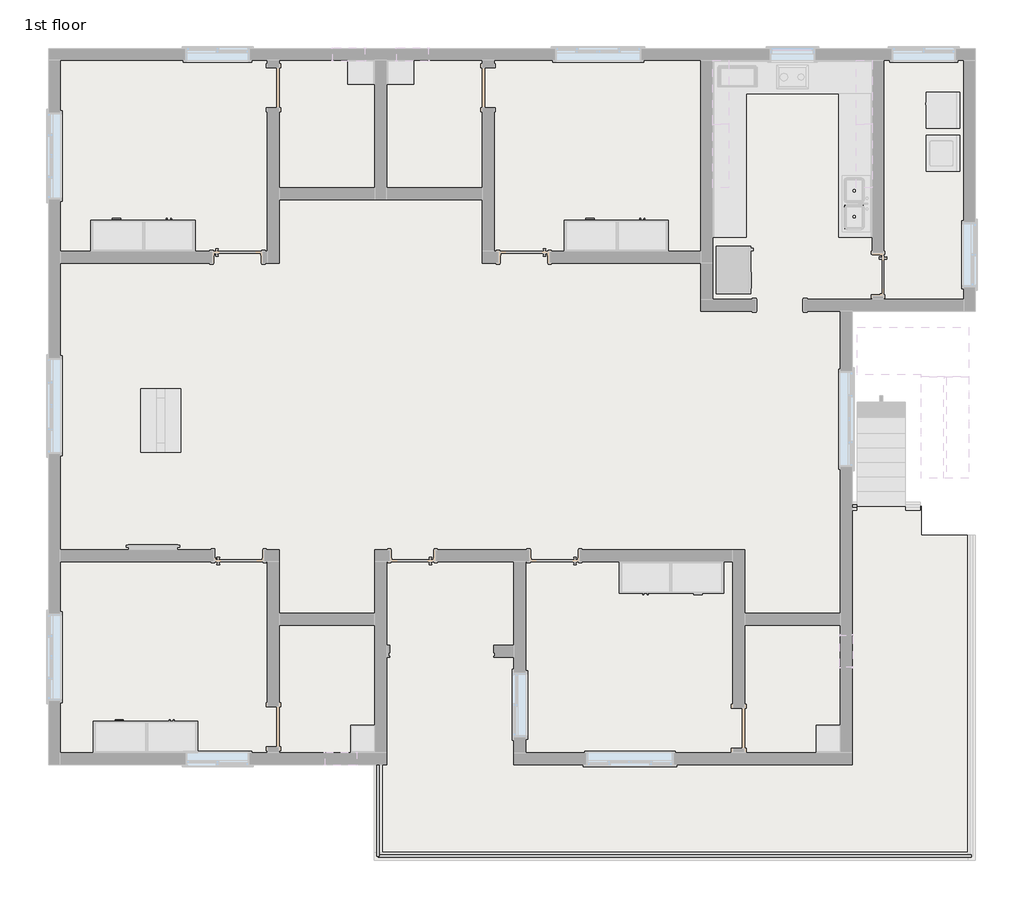
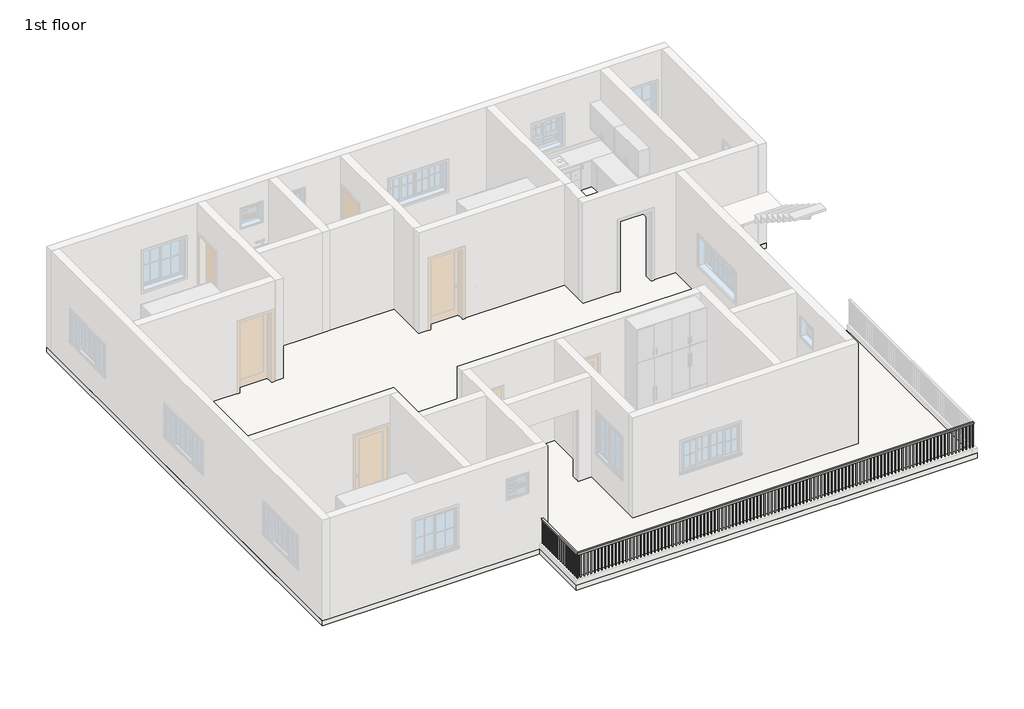
# One storey, part 2 of 4: 3 railings, 1 slab.
"""IFC4 building model written with IfcOpenShell, lengths in millimetres."""

from ifc_helpers import new_model, si_unit, frame, origin, place, context, project, spatial, polyline, outline, extrude, element, save

model = new_model("IFC4")

# Units and contexts
model_context = context("Model", 3, world=origin())
ifc_project = project(units=[si_unit("LENGTHUNIT", "METRE", prefix="MILLI")], contexts=[model_context])

# Site, building, storey
site = spatial("IfcSite", under=ifc_project)
building = spatial("IfcBuilding", under=site)
storey = spatial("IfcBuildingStorey", under=building, Name="1st floor", Elevation=3810.0)

# Railings
placement = place(None, origin())
element("IfcRailing", 1, ObjectType="Handrail - Rectangular", at=placement, inside=storey, context=model_context, shape_type="SweptSolid", body=[
    extrude(outline(polyline([(9648.8260838, -8369.2339187), (9648.8260838, -8420.0339187), (-1717.6739162, -8420.0339187), (-1717.6739162, -8369.2339187), (9648.8260838, -8369.2339187)])), frame((0.0, 0.0, 4673.6), z_axis=(0.0, 0.0, 1.0), x_axis=(1.0, 0.0, 0.0)), (0.0, 0.0, 1.0), 50.8),
    extrude(outline(polyline([(-1619.2489162, -8385.1089187), (-1619.2489162, -8404.1589187), (-1638.2989162, -8404.1589187), (-1638.2989162, -8385.1089187), (-1619.2489162, -8385.1089187)])), frame((0.0, 0.0, 3810.0), z_axis=(0.0, 0.0, 1.0), x_axis=(1.0, 0.0, 0.0)), (0.0, 0.0, 1.0), 863.6),
    extrude(outline(polyline([(-1517.6489162, -8385.1089187), (-1517.6489162, -8404.1589187), (-1536.6989162, -8404.1589187), (-1536.6989162, -8385.1089187), (-1517.6489162, -8385.1089187)])), frame((0.0, 0.0, 3810.0), z_axis=(0.0, 0.0, 1.0), x_axis=(1.0, 0.0, 0.0)), (0.0, 0.0, 1.0), 863.6),
    extrude(outline(polyline([(-1416.0489162, -8385.1089187), (-1416.0489162, -8404.1589187), (-1435.0989162, -8404.1589187), (-1435.0989162, -8385.1089187), (-1416.0489162, -8385.1089187)])), frame((0.0, 0.0, 3810.0), z_axis=(0.0, 0.0, 1.0), x_axis=(1.0, 0.0, 0.0)), (0.0, 0.0, 1.0), 863.6),
    extrude(outline(polyline([(-1314.4489162, -8385.1089187), (-1314.4489162, -8404.1589187), (-1333.4989162, -8404.1589187), (-1333.4989162, -8385.1089187), (-1314.4489162, -8385.1089187)])), frame((0.0, 0.0, 3810.0), z_axis=(0.0, 0.0, 1.0), x_axis=(1.0, 0.0, 0.0)), (0.0, 0.0, 1.0), 863.6),
    extrude(outline(polyline([(-1212.8489162, -8385.1089187), (-1212.8489162, -8404.1589187), (-1231.8989162, -8404.1589187), (-1231.8989162, -8385.1089187), (-1212.8489162, -8385.1089187)])), frame((0.0, 0.0, 3810.0), z_axis=(0.0, 0.0, 1.0), x_axis=(1.0, 0.0, 0.0)), (0.0, 0.0, 1.0), 863.6),
    extrude(outline(polyline([(-1111.2489162, -8385.1089187), (-1111.2489162, -8404.1589187), (-1130.2989162, -8404.1589187), (-1130.2989162, -8385.1089187), (-1111.2489162, -8385.1089187)])), frame((0.0, 0.0, 3810.0), z_axis=(0.0, 0.0, 1.0), x_axis=(1.0, 0.0, 0.0)), (0.0, 0.0, 1.0), 863.6),
    extrude(outline(polyline([(-1009.6489162, -8385.1089187), (-1009.6489162, -8404.1589187), (-1028.6989162, -8404.1589187), (-1028.6989162, -8385.1089187), (-1009.6489162, -8385.1089187)])), frame((0.0, 0.0, 3810.0), z_axis=(0.0, 0.0, 1.0), x_axis=(1.0, 0.0, 0.0)), (0.0, 0.0, 1.0), 863.6),
    extrude(outline(polyline([(-908.0489162, -8385.1089187), (-908.0489162, -8404.1589187), (-927.0989162, -8404.1589187), (-927.0989162, -8385.1089187), (-908.0489162, -8385.1089187)])), frame((0.0, 0.0, 3810.0), z_axis=(0.0, 0.0, 1.0), x_axis=(1.0, 0.0, 0.0)), (0.0, 0.0, 1.0), 863.6),
    extrude(outline(polyline([(-806.4489162, -8385.1089187), (-806.4489162, -8404.1589187), (-825.4989162, -8404.1589187), (-825.4989162, -8385.1089187), (-806.4489162, -8385.1089187)])), frame((0.0, 0.0, 3810.0), z_axis=(0.0, 0.0, 1.0), x_axis=(1.0, 0.0, 0.0)), (0.0, 0.0, 1.0), 863.6),
    extrude(outline(polyline([(-704.8489162, -8385.1089187), (-704.8489162, -8404.1589187), (-723.8989162, -8404.1589187), (-723.8989162, -8385.1089187), (-704.8489162, -8385.1089187)])), frame((0.0, 0.0, 3810.0), z_axis=(0.0, 0.0, 1.0), x_axis=(1.0, 0.0, 0.0)), (0.0, 0.0, 1.0), 863.6),
    extrude(outline(polyline([(-603.2489162, -8385.1089187), (-603.2489162, -8404.1589187), (-622.2989162, -8404.1589187), (-622.2989162, -8385.1089187), (-603.2489162, -8385.1089187)])), frame((0.0, 0.0, 3810.0), z_axis=(0.0, 0.0, 1.0), x_axis=(1.0, 0.0, 0.0)), (0.0, 0.0, 1.0), 863.6),
    extrude(outline(polyline([(-501.6489162, -8385.1089187), (-501.6489162, -8404.1589187), (-520.6989162, -8404.1589187), (-520.6989162, -8385.1089187), (-501.6489162, -8385.1089187)])), frame((0.0, 0.0, 3810.0), z_axis=(0.0, 0.0, 1.0), x_axis=(1.0, 0.0, 0.0)), (0.0, 0.0, 1.0), 863.6),
    extrude(outline(polyline([(-400.0489162, -8385.1089187), (-400.0489162, -8404.1589187), (-419.0989162, -8404.1589187), (-419.0989162, -8385.1089187), (-400.0489162, -8385.1089187)])), frame((0.0, 0.0, 3810.0), z_axis=(0.0, 0.0, 1.0), x_axis=(1.0, 0.0, 0.0)), (0.0, 0.0, 1.0), 863.6),
    extrude(outline(polyline([(-298.4489162, -8385.1089187), (-298.4489162, -8404.1589187), (-317.4989162, -8404.1589187), (-317.4989162, -8385.1089187), (-298.4489162, -8385.1089187)])), frame((0.0, 0.0, 3810.0), z_axis=(0.0, 0.0, 1.0), x_axis=(1.0, 0.0, 0.0)), (0.0, 0.0, 1.0), 863.6),
    extrude(outline(polyline([(-196.8489162, -8385.1089187), (-196.8489162, -8404.1589187), (-215.8989162, -8404.1589187), (-215.8989162, -8385.1089187), (-196.8489162, -8385.1089187)])), frame((0.0, 0.0, 3810.0), z_axis=(0.0, 0.0, 1.0), x_axis=(1.0, 0.0, 0.0)), (0.0, 0.0, 1.0), 863.6),
    extrude(outline(polyline([(-95.2489162, -8385.1089187), (-95.2489162, -8404.1589187), (-114.2989162, -8404.1589187), (-114.2989162, -8385.1089187), (-95.2489162, -8385.1089187)])), frame((0.0, 0.0, 3810.0), z_axis=(0.0, 0.0, 1.0), x_axis=(1.0, 0.0, 0.0)), (0.0, 0.0, 1.0), 863.6),
    extrude(outline(polyline([(6.3510838, -8385.1089187), (6.3510838, -8404.1589187), (-12.6989162, -8404.1589187), (-12.6989162, -8385.1089187), (6.3510838, -8385.1089187)])), frame((0.0, 0.0, 3810.0), z_axis=(0.0, 0.0, 1.0), x_axis=(1.0, 0.0, 0.0)), (0.0, 0.0, 1.0), 863.6),
    extrude(outline(polyline([(107.9510838, -8385.1089187), (107.9510838, -8404.1589187), (88.9010838, -8404.1589187), (88.9010838, -8385.1089187), (107.9510838, -8385.1089187)])), frame((0.0, 0.0, 3810.0), z_axis=(0.0, 0.0, 1.0), x_axis=(1.0, 0.0, 0.0)), (0.0, 0.0, 1.0), 863.6),
    extrude(outline(polyline([(209.5510838, -8385.1089187), (209.5510838, -8404.1589187), (190.5010838, -8404.1589187), (190.5010838, -8385.1089187), (209.5510838, -8385.1089187)])), frame((0.0, 0.0, 3810.0), z_axis=(0.0, 0.0, 1.0), x_axis=(1.0, 0.0, 0.0)), (0.0, 0.0, 1.0), 863.6),
    extrude(outline(polyline([(311.1510838, -8385.1089187), (311.1510838, -8404.1589187), (292.1010838, -8404.1589187), (292.1010838, -8385.1089187), (311.1510838, -8385.1089187)])), frame((0.0, 0.0, 3810.0), z_axis=(0.0, 0.0, 1.0), x_axis=(1.0, 0.0, 0.0)), (0.0, 0.0, 1.0), 863.6),
    extrude(outline(polyline([(412.7510838, -8385.1089187), (412.7510838, -8404.1589187), (393.7010838, -8404.1589187), (393.7010838, -8385.1089187), (412.7510838, -8385.1089187)])), frame((0.0, 0.0, 3810.0), z_axis=(0.0, 0.0, 1.0), x_axis=(1.0, 0.0, 0.0)), (0.0, 0.0, 1.0), 863.6),
    extrude(outline(polyline([(514.3510838, -8385.1089187), (514.3510838, -8404.1589187), (495.3010838, -8404.1589187), (495.3010838, -8385.1089187), (514.3510838, -8385.1089187)])), frame((0.0, 0.0, 3810.0), z_axis=(0.0, 0.0, 1.0), x_axis=(1.0, 0.0, 0.0)), (0.0, 0.0, 1.0), 863.6),
    extrude(outline(polyline([(615.9510838, -8385.1089187), (615.9510838, -8404.1589187), (596.9010838, -8404.1589187), (596.9010838, -8385.1089187), (615.9510838, -8385.1089187)])), frame((0.0, 0.0, 3810.0), z_axis=(0.0, 0.0, 1.0), x_axis=(1.0, 0.0, 0.0)), (0.0, 0.0, 1.0), 863.6),
    extrude(outline(polyline([(717.5510838, -8385.1089187), (717.5510838, -8404.1589187), (698.5010838, -8404.1589187), (698.5010838, -8385.1089187), (717.5510838, -8385.1089187)])), frame((0.0, 0.0, 3810.0), z_axis=(0.0, 0.0, 1.0), x_axis=(1.0, 0.0, 0.0)), (0.0, 0.0, 1.0), 863.6),
    extrude(outline(polyline([(819.1510838, -8385.1089187), (819.1510838, -8404.1589187), (800.1010838, -8404.1589187), (800.1010838, -8385.1089187), (819.1510838, -8385.1089187)])), frame((0.0, 0.0, 3810.0), z_axis=(0.0, 0.0, 1.0), x_axis=(1.0, 0.0, 0.0)), (0.0, 0.0, 1.0), 863.6),
    extrude(outline(polyline([(920.7510838, -8385.1089187), (920.7510838, -8404.1589187), (901.7010838, -8404.1589187), (901.7010838, -8385.1089187), (920.7510838, -8385.1089187)])), frame((0.0, 0.0, 3810.0), z_axis=(0.0, 0.0, 1.0), x_axis=(1.0, 0.0, 0.0)), (0.0, 0.0, 1.0), 863.6),
    extrude(outline(polyline([(1022.3510838, -8385.1089187), (1022.3510838, -8404.1589187), (1003.3010838, -8404.1589187), (1003.3010838, -8385.1089187), (1022.3510838, -8385.1089187)])), frame((0.0, 0.0, 3810.0), z_axis=(0.0, 0.0, 1.0), x_axis=(1.0, 0.0, 0.0)), (0.0, 0.0, 1.0), 863.6),
    extrude(outline(polyline([(1123.9510838, -8385.1089187), (1123.9510838, -8404.1589187), (1104.9010838, -8404.1589187), (1104.9010838, -8385.1089187), (1123.9510838, -8385.1089187)])), frame((0.0, 0.0, 3810.0), z_axis=(0.0, 0.0, 1.0), x_axis=(1.0, 0.0, 0.0)), (0.0, 0.0, 1.0), 863.6),
    extrude(outline(polyline([(1225.5510838, -8385.1089187), (1225.5510838, -8404.1589187), (1206.5010838, -8404.1589187), (1206.5010838, -8385.1089187), (1225.5510838, -8385.1089187)])), frame((0.0, 0.0, 3810.0), z_axis=(0.0, 0.0, 1.0), x_axis=(1.0, 0.0, 0.0)), (0.0, 0.0, 1.0), 863.6),
    extrude(outline(polyline([(1327.1510838, -8385.1089187), (1327.1510838, -8404.1589187), (1308.1010838, -8404.1589187), (1308.1010838, -8385.1089187), (1327.1510838, -8385.1089187)])), frame((0.0, 0.0, 3810.0), z_axis=(0.0, 0.0, 1.0), x_axis=(1.0, 0.0, 0.0)), (0.0, 0.0, 1.0), 863.6),
    extrude(outline(polyline([(1428.7510838, -8385.1089187), (1428.7510838, -8404.1589187), (1409.7010838, -8404.1589187), (1409.7010838, -8385.1089187), (1428.7510838, -8385.1089187)])), frame((0.0, 0.0, 3810.0), z_axis=(0.0, 0.0, 1.0), x_axis=(1.0, 0.0, 0.0)), (0.0, 0.0, 1.0), 863.6),
    extrude(outline(polyline([(1530.3510838, -8385.1089187), (1530.3510838, -8404.1589187), (1511.3010838, -8404.1589187), (1511.3010838, -8385.1089187), (1530.3510838, -8385.1089187)])), frame((0.0, 0.0, 3810.0), z_axis=(0.0, 0.0, 1.0), x_axis=(1.0, 0.0, 0.0)), (0.0, 0.0, 1.0), 863.6),
    extrude(outline(polyline([(1631.9510838, -8385.1089187), (1631.9510838, -8404.1589187), (1612.9010838, -8404.1589187), (1612.9010838, -8385.1089187), (1631.9510838, -8385.1089187)])), frame((0.0, 0.0, 3810.0), z_axis=(0.0, 0.0, 1.0), x_axis=(1.0, 0.0, 0.0)), (0.0, 0.0, 1.0), 863.6),
    extrude(outline(polyline([(1733.5510838, -8385.1089187), (1733.5510838, -8404.1589187), (1714.5010838, -8404.1589187), (1714.5010838, -8385.1089187), (1733.5510838, -8385.1089187)])), frame((0.0, 0.0, 3810.0), z_axis=(0.0, 0.0, 1.0), x_axis=(1.0, 0.0, 0.0)), (0.0, 0.0, 1.0), 863.6),
    extrude(outline(polyline([(1835.1510838, -8385.1089187), (1835.1510838, -8404.1589187), (1816.1010838, -8404.1589187), (1816.1010838, -8385.1089187), (1835.1510838, -8385.1089187)])), frame((0.0, 0.0, 3810.0), z_axis=(0.0, 0.0, 1.0), x_axis=(1.0, 0.0, 0.0)), (0.0, 0.0, 1.0), 863.6),
    extrude(outline(polyline([(1936.7510838, -8385.1089187), (1936.7510838, -8404.1589187), (1917.7010838, -8404.1589187), (1917.7010838, -8385.1089187), (1936.7510838, -8385.1089187)])), frame((0.0, 0.0, 3810.0), z_axis=(0.0, 0.0, 1.0), x_axis=(1.0, 0.0, 0.0)), (0.0, 0.0, 1.0), 863.6),
    extrude(outline(polyline([(2038.3510838, -8385.1089187), (2038.3510838, -8404.1589187), (2019.3010838, -8404.1589187), (2019.3010838, -8385.1089187), (2038.3510838, -8385.1089187)])), frame((0.0, 0.0, 3810.0), z_axis=(0.0, 0.0, 1.0), x_axis=(1.0, 0.0, 0.0)), (0.0, 0.0, 1.0), 863.6),
    extrude(outline(polyline([(2139.9510838, -8385.1089187), (2139.9510838, -8404.1589187), (2120.9010838, -8404.1589187), (2120.9010838, -8385.1089187), (2139.9510838, -8385.1089187)])), frame((0.0, 0.0, 3810.0), z_axis=(0.0, 0.0, 1.0), x_axis=(1.0, 0.0, 0.0)), (0.0, 0.0, 1.0), 863.6),
    extrude(outline(polyline([(2241.5510838, -8385.1089187), (2241.5510838, -8404.1589187), (2222.5010838, -8404.1589187), (2222.5010838, -8385.1089187), (2241.5510838, -8385.1089187)])), frame((0.0, 0.0, 3810.0), z_axis=(0.0, 0.0, 1.0), x_axis=(1.0, 0.0, 0.0)), (0.0, 0.0, 1.0), 863.6),
    extrude(outline(polyline([(2343.1510838, -8385.1089187), (2343.1510838, -8404.1589187), (2324.1010838, -8404.1589187), (2324.1010838, -8385.1089187), (2343.1510838, -8385.1089187)])), frame((0.0, 0.0, 3810.0), z_axis=(0.0, 0.0, 1.0), x_axis=(1.0, 0.0, 0.0)), (0.0, 0.0, 1.0), 863.6),
    extrude(outline(polyline([(2444.7510838, -8385.1089187), (2444.7510838, -8404.1589187), (2425.7010838, -8404.1589187), (2425.7010838, -8385.1089187), (2444.7510838, -8385.1089187)])), frame((0.0, 0.0, 3810.0), z_axis=(0.0, 0.0, 1.0), x_axis=(1.0, 0.0, 0.0)), (0.0, 0.0, 1.0), 863.6),
    extrude(outline(polyline([(2546.3510838, -8385.1089187), (2546.3510838, -8404.1589187), (2527.3010838, -8404.1589187), (2527.3010838, -8385.1089187), (2546.3510838, -8385.1089187)])), frame((0.0, 0.0, 3810.0), z_axis=(0.0, 0.0, 1.0), x_axis=(1.0, 0.0, 0.0)), (0.0, 0.0, 1.0), 863.6),
    extrude(outline(polyline([(2647.9510838, -8385.1089187), (2647.9510838, -8404.1589187), (2628.9010838, -8404.1589187), (2628.9010838, -8385.1089187), (2647.9510838, -8385.1089187)])), frame((0.0, 0.0, 3810.0), z_axis=(0.0, 0.0, 1.0), x_axis=(1.0, 0.0, 0.0)), (0.0, 0.0, 1.0), 863.6),
    extrude(outline(polyline([(2749.5510838, -8385.1089187), (2749.5510838, -8404.1589187), (2730.5010838, -8404.1589187), (2730.5010838, -8385.1089187), (2749.5510838, -8385.1089187)])), frame((0.0, 0.0, 3810.0), z_axis=(0.0, 0.0, 1.0), x_axis=(1.0, 0.0, 0.0)), (0.0, 0.0, 1.0), 863.6),
    extrude(outline(polyline([(2851.1510838, -8385.1089187), (2851.1510838, -8404.1589187), (2832.1010838, -8404.1589187), (2832.1010838, -8385.1089187), (2851.1510838, -8385.1089187)])), frame((0.0, 0.0, 3810.0), z_axis=(0.0, 0.0, 1.0), x_axis=(1.0, 0.0, 0.0)), (0.0, 0.0, 1.0), 863.6),
    extrude(outline(polyline([(2952.7510838, -8385.1089187), (2952.7510838, -8404.1589187), (2933.7010838, -8404.1589187), (2933.7010838, -8385.1089187), (2952.7510838, -8385.1089187)])), frame((0.0, 0.0, 3810.0), z_axis=(0.0, 0.0, 1.0), x_axis=(1.0, 0.0, 0.0)), (0.0, 0.0, 1.0), 863.6),
    extrude(outline(polyline([(3054.3510838, -8385.1089187), (3054.3510838, -8404.1589187), (3035.3010838, -8404.1589187), (3035.3010838, -8385.1089187), (3054.3510838, -8385.1089187)])), frame((0.0, 0.0, 3810.0), z_axis=(0.0, 0.0, 1.0), x_axis=(1.0, 0.0, 0.0)), (0.0, 0.0, 1.0), 863.6),
    extrude(outline(polyline([(3155.9510838, -8385.1089187), (3155.9510838, -8404.1589187), (3136.9010838, -8404.1589187), (3136.9010838, -8385.1089187), (3155.9510838, -8385.1089187)])), frame((0.0, 0.0, 3810.0), z_axis=(0.0, 0.0, 1.0), x_axis=(1.0, 0.0, 0.0)), (0.0, 0.0, 1.0), 863.6),
    extrude(outline(polyline([(3257.5510838, -8385.1089187), (3257.5510838, -8404.1589187), (3238.5010838, -8404.1589187), (3238.5010838, -8385.1089187), (3257.5510838, -8385.1089187)])), frame((0.0, 0.0, 3810.0), z_axis=(0.0, 0.0, 1.0), x_axis=(1.0, 0.0, 0.0)), (0.0, 0.0, 1.0), 863.6),
    extrude(outline(polyline([(3359.1510838, -8385.1089187), (3359.1510838, -8404.1589187), (3340.1010838, -8404.1589187), (3340.1010838, -8385.1089187), (3359.1510838, -8385.1089187)])), frame((0.0, 0.0, 3810.0), z_axis=(0.0, 0.0, 1.0), x_axis=(1.0, 0.0, 0.0)), (0.0, 0.0, 1.0), 863.6),
    extrude(outline(polyline([(3460.7510838, -8385.1089187), (3460.7510838, -8404.1589187), (3441.7010838, -8404.1589187), (3441.7010838, -8385.1089187), (3460.7510838, -8385.1089187)])), frame((0.0, 0.0, 3810.0), z_axis=(0.0, 0.0, 1.0), x_axis=(1.0, 0.0, 0.0)), (0.0, 0.0, 1.0), 863.6),
    extrude(outline(polyline([(3562.3510838, -8385.1089187), (3562.3510838, -8404.1589187), (3543.3010838, -8404.1589187), (3543.3010838, -8385.1089187), (3562.3510838, -8385.1089187)])), frame((0.0, 0.0, 3810.0), z_axis=(0.0, 0.0, 1.0), x_axis=(1.0, 0.0, 0.0)), (0.0, 0.0, 1.0), 863.6),
    extrude(outline(polyline([(3663.9510838, -8385.1089187), (3663.9510838, -8404.1589187), (3644.9010838, -8404.1589187), (3644.9010838, -8385.1089187), (3663.9510838, -8385.1089187)])), frame((0.0, 0.0, 3810.0), z_axis=(0.0, 0.0, 1.0), x_axis=(1.0, 0.0, 0.0)), (0.0, 0.0, 1.0), 863.6),
    extrude(outline(polyline([(3765.5510838, -8385.1089187), (3765.5510838, -8404.1589187), (3746.5010838, -8404.1589187), (3746.5010838, -8385.1089187), (3765.5510838, -8385.1089187)])), frame((0.0, 0.0, 3810.0), z_axis=(0.0, 0.0, 1.0), x_axis=(1.0, 0.0, 0.0)), (0.0, 0.0, 1.0), 863.6),
    extrude(outline(polyline([(3867.1510838, -8385.1089187), (3867.1510838, -8404.1589187), (3848.1010838, -8404.1589187), (3848.1010838, -8385.1089187), (3867.1510838, -8385.1089187)])), frame((0.0, 0.0, 3810.0), z_axis=(0.0, 0.0, 1.0), x_axis=(1.0, 0.0, 0.0)), (0.0, 0.0, 1.0), 863.6),
    extrude(outline(polyline([(3968.7510838, -8385.1089187), (3968.7510838, -8404.1589187), (3949.7010838, -8404.1589187), (3949.7010838, -8385.1089187), (3968.7510838, -8385.1089187)])), frame((0.0, 0.0, 3810.0), z_axis=(0.0, 0.0, 1.0), x_axis=(1.0, 0.0, 0.0)), (0.0, 0.0, 1.0), 863.6),
    extrude(outline(polyline([(4070.3510838, -8385.1089187), (4070.3510838, -8404.1589187), (4051.3010838, -8404.1589187), (4051.3010838, -8385.1089187), (4070.3510838, -8385.1089187)])), frame((0.0, 0.0, 3810.0), z_axis=(0.0, 0.0, 1.0), x_axis=(1.0, 0.0, 0.0)), (0.0, 0.0, 1.0), 863.6),
    extrude(outline(polyline([(4171.9510838, -8385.1089187), (4171.9510838, -8404.1589187), (4152.9010838, -8404.1589187), (4152.9010838, -8385.1089187), (4171.9510838, -8385.1089187)])), frame((0.0, 0.0, 3810.0), z_axis=(0.0, 0.0, 1.0), x_axis=(1.0, 0.0, 0.0)), (0.0, 0.0, 1.0), 863.6),
    extrude(outline(polyline([(4273.5510838, -8385.1089187), (4273.5510838, -8404.1589187), (4254.5010838, -8404.1589187), (4254.5010838, -8385.1089187), (4273.5510838, -8385.1089187)])), frame((0.0, 0.0, 3810.0), z_axis=(0.0, 0.0, 1.0), x_axis=(1.0, 0.0, 0.0)), (0.0, 0.0, 1.0), 863.6),
    extrude(outline(polyline([(4375.1510838, -8385.1089187), (4375.1510838, -8404.1589187), (4356.1010838, -8404.1589187), (4356.1010838, -8385.1089187), (4375.1510838, -8385.1089187)])), frame((0.0, 0.0, 3810.0), z_axis=(0.0, 0.0, 1.0), x_axis=(1.0, 0.0, 0.0)), (0.0, 0.0, 1.0), 863.6),
    extrude(outline(polyline([(4476.7510838, -8385.1089187), (4476.7510838, -8404.1589187), (4457.7010838, -8404.1589187), (4457.7010838, -8385.1089187), (4476.7510838, -8385.1089187)])), frame((0.0, 0.0, 3810.0), z_axis=(0.0, 0.0, 1.0), x_axis=(1.0, 0.0, 0.0)), (0.0, 0.0, 1.0), 863.6),
    extrude(outline(polyline([(4578.3510838, -8385.1089187), (4578.3510838, -8404.1589187), (4559.3010838, -8404.1589187), (4559.3010838, -8385.1089187), (4578.3510838, -8385.1089187)])), frame((0.0, 0.0, 3810.0), z_axis=(0.0, 0.0, 1.0), x_axis=(1.0, 0.0, 0.0)), (0.0, 0.0, 1.0), 863.6),
    extrude(outline(polyline([(4679.9510838, -8385.1089187), (4679.9510838, -8404.1589187), (4660.9010838, -8404.1589187), (4660.9010838, -8385.1089187), (4679.9510838, -8385.1089187)])), frame((0.0, 0.0, 3810.0), z_axis=(0.0, 0.0, 1.0), x_axis=(1.0, 0.0, 0.0)), (0.0, 0.0, 1.0), 863.6),
    extrude(outline(polyline([(4781.5510838, -8385.1089187), (4781.5510838, -8404.1589187), (4762.5010838, -8404.1589187), (4762.5010838, -8385.1089187), (4781.5510838, -8385.1089187)])), frame((0.0, 0.0, 3810.0), z_axis=(0.0, 0.0, 1.0), x_axis=(1.0, 0.0, 0.0)), (0.0, 0.0, 1.0), 863.6),
    extrude(outline(polyline([(4883.1510838, -8385.1089187), (4883.1510838, -8404.1589187), (4864.1010838, -8404.1589187), (4864.1010838, -8385.1089187), (4883.1510838, -8385.1089187)])), frame((0.0, 0.0, 3810.0), z_axis=(0.0, 0.0, 1.0), x_axis=(1.0, 0.0, 0.0)), (0.0, 0.0, 1.0), 863.6),
    extrude(outline(polyline([(4984.7510838, -8385.1089187), (4984.7510838, -8404.1589187), (4965.7010838, -8404.1589187), (4965.7010838, -8385.1089187), (4984.7510838, -8385.1089187)])), frame((0.0, 0.0, 3810.0), z_axis=(0.0, 0.0, 1.0), x_axis=(1.0, 0.0, 0.0)), (0.0, 0.0, 1.0), 863.6),
    extrude(outline(polyline([(5086.3510838, -8385.1089187), (5086.3510838, -8404.1589187), (5067.3010838, -8404.1589187), (5067.3010838, -8385.1089187), (5086.3510838, -8385.1089187)])), frame((0.0, 0.0, 3810.0), z_axis=(0.0, 0.0, 1.0), x_axis=(1.0, 0.0, 0.0)), (0.0, 0.0, 1.0), 863.6),
    extrude(outline(polyline([(5187.9510838, -8385.1089187), (5187.9510838, -8404.1589187), (5168.9010838, -8404.1589187), (5168.9010838, -8385.1089187), (5187.9510838, -8385.1089187)])), frame((0.0, 0.0, 3810.0), z_axis=(0.0, 0.0, 1.0), x_axis=(1.0, 0.0, 0.0)), (0.0, 0.0, 1.0), 863.6),
    extrude(outline(polyline([(5289.5510838, -8385.1089187), (5289.5510838, -8404.1589187), (5270.5010838, -8404.1589187), (5270.5010838, -8385.1089187), (5289.5510838, -8385.1089187)])), frame((0.0, 0.0, 3810.0), z_axis=(0.0, 0.0, 1.0), x_axis=(1.0, 0.0, 0.0)), (0.0, 0.0, 1.0), 863.6),
    extrude(outline(polyline([(5391.1510838, -8385.1089187), (5391.1510838, -8404.1589187), (5372.1010838, -8404.1589187), (5372.1010838, -8385.1089187), (5391.1510838, -8385.1089187)])), frame((0.0, 0.0, 3810.0), z_axis=(0.0, 0.0, 1.0), x_axis=(1.0, 0.0, 0.0)), (0.0, 0.0, 1.0), 863.6),
    extrude(outline(polyline([(5492.7510838, -8385.1089187), (5492.7510838, -8404.1589187), (5473.7010838, -8404.1589187), (5473.7010838, -8385.1089187), (5492.7510838, -8385.1089187)])), frame((0.0, 0.0, 3810.0), z_axis=(0.0, 0.0, 1.0), x_axis=(1.0, 0.0, 0.0)), (0.0, 0.0, 1.0), 863.6),
    extrude(outline(polyline([(5594.3510838, -8385.1089187), (5594.3510838, -8404.1589187), (5575.3010838, -8404.1589187), (5575.3010838, -8385.1089187), (5594.3510838, -8385.1089187)])), frame((0.0, 0.0, 3810.0), z_axis=(0.0, 0.0, 1.0), x_axis=(1.0, 0.0, 0.0)), (0.0, 0.0, 1.0), 863.6),
    extrude(outline(polyline([(5695.9510838, -8385.1089187), (5695.9510838, -8404.1589187), (5676.9010838, -8404.1589187), (5676.9010838, -8385.1089187), (5695.9510838, -8385.1089187)])), frame((0.0, 0.0, 3810.0), z_axis=(0.0, 0.0, 1.0), x_axis=(1.0, 0.0, 0.0)), (0.0, 0.0, 1.0), 863.6),
    extrude(outline(polyline([(5797.5510838, -8385.1089187), (5797.5510838, -8404.1589187), (5778.5010838, -8404.1589187), (5778.5010838, -8385.1089187), (5797.5510838, -8385.1089187)])), frame((0.0, 0.0, 3810.0), z_axis=(0.0, 0.0, 1.0), x_axis=(1.0, 0.0, 0.0)), (0.0, 0.0, 1.0), 863.6),
    extrude(outline(polyline([(5899.1510838, -8385.1089187), (5899.1510838, -8404.1589187), (5880.1010838, -8404.1589187), (5880.1010838, -8385.1089187), (5899.1510838, -8385.1089187)])), frame((0.0, 0.0, 3810.0), z_axis=(0.0, 0.0, 1.0), x_axis=(1.0, 0.0, 0.0)), (0.0, 0.0, 1.0), 863.6),
    extrude(outline(polyline([(6000.7510838, -8385.1089187), (6000.7510838, -8404.1589187), (5981.7010838, -8404.1589187), (5981.7010838, -8385.1089187), (6000.7510838, -8385.1089187)])), frame((0.0, 0.0, 3810.0), z_axis=(0.0, 0.0, 1.0), x_axis=(1.0, 0.0, 0.0)), (0.0, 0.0, 1.0), 863.6),
    extrude(outline(polyline([(6102.3510838, -8385.1089187), (6102.3510838, -8404.1589187), (6083.3010838, -8404.1589187), (6083.3010838, -8385.1089187), (6102.3510838, -8385.1089187)])), frame((0.0, 0.0, 3810.0), z_axis=(0.0, 0.0, 1.0), x_axis=(1.0, 0.0, 0.0)), (0.0, 0.0, 1.0), 863.6),
    extrude(outline(polyline([(6203.9510838, -8385.1089187), (6203.9510838, -8404.1589187), (6184.9010838, -8404.1589187), (6184.9010838, -8385.1089187), (6203.9510838, -8385.1089187)])), frame((0.0, 0.0, 3810.0), z_axis=(0.0, 0.0, 1.0), x_axis=(1.0, 0.0, 0.0)), (0.0, 0.0, 1.0), 863.6),
    extrude(outline(polyline([(6305.5510838, -8385.1089187), (6305.5510838, -8404.1589187), (6286.5010838, -8404.1589187), (6286.5010838, -8385.1089187), (6305.5510838, -8385.1089187)])), frame((0.0, 0.0, 3810.0), z_axis=(0.0, 0.0, 1.0), x_axis=(1.0, 0.0, 0.0)), (0.0, 0.0, 1.0), 863.6),
    extrude(outline(polyline([(6407.1510838, -8385.1089187), (6407.1510838, -8404.1589187), (6388.1010838, -8404.1589187), (6388.1010838, -8385.1089187), (6407.1510838, -8385.1089187)])), frame((0.0, 0.0, 3810.0), z_axis=(0.0, 0.0, 1.0), x_axis=(1.0, 0.0, 0.0)), (0.0, 0.0, 1.0), 863.6),
    extrude(outline(polyline([(6508.7510838, -8385.1089187), (6508.7510838, -8404.1589187), (6489.7010838, -8404.1589187), (6489.7010838, -8385.1089187), (6508.7510838, -8385.1089187)])), frame((0.0, 0.0, 3810.0), z_axis=(0.0, 0.0, 1.0), x_axis=(1.0, 0.0, 0.0)), (0.0, 0.0, 1.0), 863.6),
    extrude(outline(polyline([(6610.3510838, -8385.1089187), (6610.3510838, -8404.1589187), (6591.3010838, -8404.1589187), (6591.3010838, -8385.1089187), (6610.3510838, -8385.1089187)])), frame((0.0, 0.0, 3810.0), z_axis=(0.0, 0.0, 1.0), x_axis=(1.0, 0.0, 0.0)), (0.0, 0.0, 1.0), 863.6),
    extrude(outline(polyline([(6711.9510838, -8385.1089187), (6711.9510838, -8404.1589187), (6692.9010838, -8404.1589187), (6692.9010838, -8385.1089187), (6711.9510838, -8385.1089187)])), frame((0.0, 0.0, 3810.0), z_axis=(0.0, 0.0, 1.0), x_axis=(1.0, 0.0, 0.0)), (0.0, 0.0, 1.0), 863.6),
    extrude(outline(polyline([(6813.5510838, -8385.1089187), (6813.5510838, -8404.1589187), (6794.5010838, -8404.1589187), (6794.5010838, -8385.1089187), (6813.5510838, -8385.1089187)])), frame((0.0, 0.0, 3810.0), z_axis=(0.0, 0.0, 1.0), x_axis=(1.0, 0.0, 0.0)), (0.0, 0.0, 1.0), 863.6),
    extrude(outline(polyline([(6915.1510838, -8385.1089187), (6915.1510838, -8404.1589187), (6896.1010838, -8404.1589187), (6896.1010838, -8385.1089187), (6915.1510838, -8385.1089187)])), frame((0.0, 0.0, 3810.0), z_axis=(0.0, 0.0, 1.0), x_axis=(1.0, 0.0, 0.0)), (0.0, 0.0, 1.0), 863.6),
    extrude(outline(polyline([(7016.7510838, -8385.1089187), (7016.7510838, -8404.1589187), (6997.7010838, -8404.1589187), (6997.7010838, -8385.1089187), (7016.7510838, -8385.1089187)])), frame((0.0, 0.0, 3810.0), z_axis=(0.0, 0.0, 1.0), x_axis=(1.0, 0.0, 0.0)), (0.0, 0.0, 1.0), 863.6),
    extrude(outline(polyline([(7118.3510838, -8385.1089187), (7118.3510838, -8404.1589187), (7099.3010838, -8404.1589187), (7099.3010838, -8385.1089187), (7118.3510838, -8385.1089187)])), frame((0.0, 0.0, 3810.0), z_axis=(0.0, 0.0, 1.0), x_axis=(1.0, 0.0, 0.0)), (0.0, 0.0, 1.0), 863.6),
    extrude(outline(polyline([(7219.9510838, -8385.1089187), (7219.9510838, -8404.1589187), (7200.9010838, -8404.1589187), (7200.9010838, -8385.1089187), (7219.9510838, -8385.1089187)])), frame((0.0, 0.0, 3810.0), z_axis=(0.0, 0.0, 1.0), x_axis=(1.0, 0.0, 0.0)), (0.0, 0.0, 1.0), 863.6),
    extrude(outline(polyline([(7321.5510838, -8385.1089187), (7321.5510838, -8404.1589187), (7302.5010838, -8404.1589187), (7302.5010838, -8385.1089187), (7321.5510838, -8385.1089187)])), frame((0.0, 0.0, 3810.0), z_axis=(0.0, 0.0, 1.0), x_axis=(1.0, 0.0, 0.0)), (0.0, 0.0, 1.0), 863.6),
    extrude(outline(polyline([(7423.1510838, -8385.1089187), (7423.1510838, -8404.1589187), (7404.1010838, -8404.1589187), (7404.1010838, -8385.1089187), (7423.1510838, -8385.1089187)])), frame((0.0, 0.0, 3810.0), z_axis=(0.0, 0.0, 1.0), x_axis=(1.0, 0.0, 0.0)), (0.0, 0.0, 1.0), 863.6),
    extrude(outline(polyline([(7524.7510838, -8385.1089187), (7524.7510838, -8404.1589187), (7505.7010838, -8404.1589187), (7505.7010838, -8385.1089187), (7524.7510838, -8385.1089187)])), frame((0.0, 0.0, 3810.0), z_axis=(0.0, 0.0, 1.0), x_axis=(1.0, 0.0, 0.0)), (0.0, 0.0, 1.0), 863.6),
    extrude(outline(polyline([(7626.3510838, -8385.1089187), (7626.3510838, -8404.1589187), (7607.3010838, -8404.1589187), (7607.3010838, -8385.1089187), (7626.3510838, -8385.1089187)])), frame((0.0, 0.0, 3810.0), z_axis=(0.0, 0.0, 1.0), x_axis=(1.0, 0.0, 0.0)), (0.0, 0.0, 1.0), 863.6),
    extrude(outline(polyline([(7727.9510838, -8385.1089187), (7727.9510838, -8404.1589187), (7708.9010838, -8404.1589187), (7708.9010838, -8385.1089187), (7727.9510838, -8385.1089187)])), frame((0.0, 0.0, 3810.0), z_axis=(0.0, 0.0, 1.0), x_axis=(1.0, 0.0, 0.0)), (0.0, 0.0, 1.0), 863.6),
    extrude(outline(polyline([(7829.5510838, -8385.1089187), (7829.5510838, -8404.1589187), (7810.5010838, -8404.1589187), (7810.5010838, -8385.1089187), (7829.5510838, -8385.1089187)])), frame((0.0, 0.0, 3810.0), z_axis=(0.0, 0.0, 1.0), x_axis=(1.0, 0.0, 0.0)), (0.0, 0.0, 1.0), 863.6),
    extrude(outline(polyline([(7931.1510838, -8385.1089187), (7931.1510838, -8404.1589187), (7912.1010838, -8404.1589187), (7912.1010838, -8385.1089187), (7931.1510838, -8385.1089187)])), frame((0.0, 0.0, 3810.0), z_axis=(0.0, 0.0, 1.0), x_axis=(1.0, 0.0, 0.0)), (0.0, 0.0, 1.0), 863.6),
    extrude(outline(polyline([(8032.7510838, -8385.1089187), (8032.7510838, -8404.1589187), (8013.7010838, -8404.1589187), (8013.7010838, -8385.1089187), (8032.7510838, -8385.1089187)])), frame((0.0, 0.0, 3810.0), z_axis=(0.0, 0.0, 1.0), x_axis=(1.0, 0.0, 0.0)), (0.0, 0.0, 1.0), 863.6),
    extrude(outline(polyline([(8134.3510838, -8385.1089187), (8134.3510838, -8404.1589187), (8115.3010838, -8404.1589187), (8115.3010838, -8385.1089187), (8134.3510838, -8385.1089187)])), frame((0.0, 0.0, 3810.0), z_axis=(0.0, 0.0, 1.0), x_axis=(1.0, 0.0, 0.0)), (0.0, 0.0, 1.0), 863.6),
    extrude(outline(polyline([(8235.9510838, -8385.1089187), (8235.9510838, -8404.1589187), (8216.9010838, -8404.1589187), (8216.9010838, -8385.1089187), (8235.9510838, -8385.1089187)])), frame((0.0, 0.0, 3810.0), z_axis=(0.0, 0.0, 1.0), x_axis=(1.0, 0.0, 0.0)), (0.0, 0.0, 1.0), 863.6),
    extrude(outline(polyline([(8337.5510838, -8385.1089187), (8337.5510838, -8404.1589187), (8318.5010838, -8404.1589187), (8318.5010838, -8385.1089187), (8337.5510838, -8385.1089187)])), frame((0.0, 0.0, 3810.0), z_axis=(0.0, 0.0, 1.0), x_axis=(1.0, 0.0, 0.0)), (0.0, 0.0, 1.0), 863.6),
    extrude(outline(polyline([(8439.1510838, -8385.1089187), (8439.1510838, -8404.1589187), (8420.1010838, -8404.1589187), (8420.1010838, -8385.1089187), (8439.1510838, -8385.1089187)])), frame((0.0, 0.0, 3810.0), z_axis=(0.0, 0.0, 1.0), x_axis=(1.0, 0.0, 0.0)), (0.0, 0.0, 1.0), 863.6),
    extrude(outline(polyline([(8540.7510838, -8385.1089187), (8540.7510838, -8404.1589187), (8521.7010838, -8404.1589187), (8521.7010838, -8385.1089187), (8540.7510838, -8385.1089187)])), frame((0.0, 0.0, 3810.0), z_axis=(0.0, 0.0, 1.0), x_axis=(1.0, 0.0, 0.0)), (0.0, 0.0, 1.0), 863.6),
    extrude(outline(polyline([(8642.3510838, -8385.1089187), (8642.3510838, -8404.1589187), (8623.3010838, -8404.1589187), (8623.3010838, -8385.1089187), (8642.3510838, -8385.1089187)])), frame((0.0, 0.0, 3810.0), z_axis=(0.0, 0.0, 1.0), x_axis=(1.0, 0.0, 0.0)), (0.0, 0.0, 1.0), 863.6),
    extrude(outline(polyline([(8743.9510838, -8385.1089187), (8743.9510838, -8404.1589187), (8724.9010838, -8404.1589187), (8724.9010838, -8385.1089187), (8743.9510838, -8385.1089187)])), frame((0.0, 0.0, 3810.0), z_axis=(0.0, 0.0, 1.0), x_axis=(1.0, 0.0, 0.0)), (0.0, 0.0, 1.0), 863.6),
    extrude(outline(polyline([(8845.5510838, -8385.1089187), (8845.5510838, -8404.1589187), (8826.5010838, -8404.1589187), (8826.5010838, -8385.1089187), (8845.5510838, -8385.1089187)])), frame((0.0, 0.0, 3810.0), z_axis=(0.0, 0.0, 1.0), x_axis=(1.0, 0.0, 0.0)), (0.0, 0.0, 1.0), 863.6),
    extrude(outline(polyline([(8947.1510838, -8385.1089187), (8947.1510838, -8404.1589187), (8928.1010838, -8404.1589187), (8928.1010838, -8385.1089187), (8947.1510838, -8385.1089187)])), frame((0.0, 0.0, 3810.0), z_axis=(0.0, 0.0, 1.0), x_axis=(1.0, 0.0, 0.0)), (0.0, 0.0, 1.0), 863.6),
    extrude(outline(polyline([(9048.7510838, -8385.1089187), (9048.7510838, -8404.1589187), (9029.7010838, -8404.1589187), (9029.7010838, -8385.1089187), (9048.7510838, -8385.1089187)])), frame((0.0, 0.0, 3810.0), z_axis=(0.0, 0.0, 1.0), x_axis=(1.0, 0.0, 0.0)), (0.0, 0.0, 1.0), 863.6),
    extrude(outline(polyline([(9150.3510838, -8385.1089187), (9150.3510838, -8404.1589187), (9131.3010838, -8404.1589187), (9131.3010838, -8385.1089187), (9150.3510838, -8385.1089187)])), frame((0.0, 0.0, 3810.0), z_axis=(0.0, 0.0, 1.0), x_axis=(1.0, 0.0, 0.0)), (0.0, 0.0, 1.0), 863.6),
    extrude(outline(polyline([(9251.9510838, -8385.1089187), (9251.9510838, -8404.1589187), (9232.9010838, -8404.1589187), (9232.9010838, -8385.1089187), (9251.9510838, -8385.1089187)])), frame((0.0, 0.0, 3810.0), z_axis=(0.0, 0.0, 1.0), x_axis=(1.0, 0.0, 0.0)), (0.0, 0.0, 1.0), 863.6),
    extrude(outline(polyline([(9353.5510838, -8385.1089187), (9353.5510838, -8404.1589187), (9334.5010838, -8404.1589187), (9334.5010838, -8385.1089187), (9353.5510838, -8385.1089187)])), frame((0.0, 0.0, 3810.0), z_axis=(0.0, 0.0, 1.0), x_axis=(1.0, 0.0, 0.0)), (0.0, 0.0, 1.0), 863.6),
    extrude(outline(polyline([(9455.1510838, -8385.1089187), (9455.1510838, -8404.1589187), (9436.1010838, -8404.1589187), (9436.1010838, -8385.1089187), (9455.1510838, -8385.1089187)])), frame((0.0, 0.0, 3810.0), z_axis=(0.0, 0.0, 1.0), x_axis=(1.0, 0.0, 0.0)), (0.0, 0.0, 1.0), 863.6),
    extrude(outline(polyline([(9556.7510838, -8385.1089187), (9556.7510838, -8404.1589187), (9537.7010838, -8404.1589187), (9537.7010838, -8385.1089187), (9556.7510838, -8385.1089187)])), frame((0.0, 0.0, 3810.0), z_axis=(0.0, 0.0, 1.0), x_axis=(1.0, 0.0, 0.0)), (0.0, 0.0, 1.0), 863.6),
    extrude(outline(polyline([(-1698.6239162, -8385.1089187), (-1698.6239162, -8404.1589187), (-1717.6739162, -8404.1589187), (-1717.6739162, -8385.1089187), (-1698.6239162, -8385.1089187)])), frame((0.0, 0.0, 3810.0), z_axis=(0.0, 0.0, 1.0), x_axis=(1.0, 0.0, 0.0)), (0.0, 0.0, 1.0), 863.6),
    extrude(outline(polyline([(9648.8260838, -8385.1089187), (9648.8260838, -8404.1589187), (9629.7760838, -8404.1589187), (9629.7760838, -8385.1089187), (9648.8260838, -8385.1089187)])), frame((0.0, 0.0, 3810.0), z_axis=(0.0, 0.0, 1.0), x_axis=(1.0, 0.0, 0.0)), (0.0, 0.0, 1.0), 863.6),
])
element("IfcRailing", 2, ObjectType="Handrail - Rectangular", at=placement, inside=storey, context=model_context, shape_type="SweptSolid", body=[
    extrude(outline(polyline([(-1743.0739162, -6642.0339187), (-1692.2739162, -6642.0339187), (-1692.2739162, -8394.6339187), (-1743.0739162, -8394.6339187), (-1743.0739162, -6642.0339187)])), frame((0.0, 0.0, 4673.6), z_axis=(0.0, 0.0, 1.0), x_axis=(1.0, 0.0, 0.0)), (0.0, 0.0, 1.0), 50.8),
    extrude(outline(polyline([(-1727.1989162, -8359.7089187), (-1708.1489162, -8359.7089187), (-1708.1489162, -8378.7589187), (-1727.1989162, -8378.7589187), (-1727.1989162, -8359.7089187)])), frame((0.0, 0.0, 3810.0), z_axis=(0.0, 0.0, 1.0), x_axis=(1.0, 0.0, 0.0)), (0.0, 0.0, 1.0), 863.6),
    extrude(outline(polyline([(-1727.1989162, -8258.1089187), (-1708.1489162, -8258.1089187), (-1708.1489162, -8277.1589187), (-1727.1989162, -8277.1589187), (-1727.1989162, -8258.1089187)])), frame((0.0, 0.0, 3810.0), z_axis=(0.0, 0.0, 1.0), x_axis=(1.0, 0.0, 0.0)), (0.0, 0.0, 1.0), 863.6),
    extrude(outline(polyline([(-1727.1989162, -8156.5089187), (-1708.1489162, -8156.5089187), (-1708.1489162, -8175.5589187), (-1727.1989162, -8175.5589187), (-1727.1989162, -8156.5089187)])), frame((0.0, 0.0, 3810.0), z_axis=(0.0, 0.0, 1.0), x_axis=(1.0, 0.0, 0.0)), (0.0, 0.0, 1.0), 863.6),
    extrude(outline(polyline([(-1727.1989162, -8054.9089187), (-1708.1489162, -8054.9089187), (-1708.1489162, -8073.9589187), (-1727.1989162, -8073.9589187), (-1727.1989162, -8054.9089187)])), frame((0.0, 0.0, 3810.0), z_axis=(0.0, 0.0, 1.0), x_axis=(1.0, 0.0, 0.0)), (0.0, 0.0, 1.0), 863.6),
    extrude(outline(polyline([(-1727.1989162, -7953.3089187), (-1708.1489162, -7953.3089187), (-1708.1489162, -7972.3589187), (-1727.1989162, -7972.3589187), (-1727.1989162, -7953.3089187)])), frame((0.0, 0.0, 3810.0), z_axis=(0.0, 0.0, 1.0), x_axis=(1.0, 0.0, 0.0)), (0.0, 0.0, 1.0), 863.6),
    extrude(outline(polyline([(-1727.1989162, -7851.7089187), (-1708.1489162, -7851.7089187), (-1708.1489162, -7870.7589187), (-1727.1989162, -7870.7589187), (-1727.1989162, -7851.7089187)])), frame((0.0, 0.0, 3810.0), z_axis=(0.0, 0.0, 1.0), x_axis=(1.0, 0.0, 0.0)), (0.0, 0.0, 1.0), 863.6),
    extrude(outline(polyline([(-1727.1989162, -7750.1089187), (-1708.1489162, -7750.1089187), (-1708.1489162, -7769.1589187), (-1727.1989162, -7769.1589187), (-1727.1989162, -7750.1089187)])), frame((0.0, 0.0, 3810.0), z_axis=(0.0, 0.0, 1.0), x_axis=(1.0, 0.0, 0.0)), (0.0, 0.0, 1.0), 863.6),
    extrude(outline(polyline([(-1727.1989162, -7648.5089187), (-1708.1489162, -7648.5089187), (-1708.1489162, -7667.5589187), (-1727.1989162, -7667.5589187), (-1727.1989162, -7648.5089187)])), frame((0.0, 0.0, 3810.0), z_axis=(0.0, 0.0, 1.0), x_axis=(1.0, 0.0, 0.0)), (0.0, 0.0, 1.0), 863.6),
    extrude(outline(polyline([(-1727.1989162, -7546.9089187), (-1708.1489162, -7546.9089187), (-1708.1489162, -7565.9589187), (-1727.1989162, -7565.9589187), (-1727.1989162, -7546.9089187)])), frame((0.0, 0.0, 3810.0), z_axis=(0.0, 0.0, 1.0), x_axis=(1.0, 0.0, 0.0)), (0.0, 0.0, 1.0), 863.6),
    extrude(outline(polyline([(-1727.1989162, -7445.3089187), (-1708.1489162, -7445.3089187), (-1708.1489162, -7464.3589187), (-1727.1989162, -7464.3589187), (-1727.1989162, -7445.3089187)])), frame((0.0, 0.0, 3810.0), z_axis=(0.0, 0.0, 1.0), x_axis=(1.0, 0.0, 0.0)), (0.0, 0.0, 1.0), 863.6),
    extrude(outline(polyline([(-1727.1989162, -7343.7089187), (-1708.1489162, -7343.7089187), (-1708.1489162, -7362.7589187), (-1727.1989162, -7362.7589187), (-1727.1989162, -7343.7089187)])), frame((0.0, 0.0, 3810.0), z_axis=(0.0, 0.0, 1.0), x_axis=(1.0, 0.0, 0.0)), (0.0, 0.0, 1.0), 863.6),
    extrude(outline(polyline([(-1727.1989162, -7242.1089187), (-1708.1489162, -7242.1089187), (-1708.1489162, -7261.1589187), (-1727.1989162, -7261.1589187), (-1727.1989162, -7242.1089187)])), frame((0.0, 0.0, 3810.0), z_axis=(0.0, 0.0, 1.0), x_axis=(1.0, 0.0, 0.0)), (0.0, 0.0, 1.0), 863.6),
    extrude(outline(polyline([(-1727.1989162, -7140.5089187), (-1708.1489162, -7140.5089187), (-1708.1489162, -7159.5589187), (-1727.1989162, -7159.5589187), (-1727.1989162, -7140.5089187)])), frame((0.0, 0.0, 3810.0), z_axis=(0.0, 0.0, 1.0), x_axis=(1.0, 0.0, 0.0)), (0.0, 0.0, 1.0), 863.6),
    extrude(outline(polyline([(-1727.1989162, -7038.9089187), (-1708.1489162, -7038.9089187), (-1708.1489162, -7057.9589187), (-1727.1989162, -7057.9589187), (-1727.1989162, -7038.9089187)])), frame((0.0, 0.0, 3810.0), z_axis=(0.0, 0.0, 1.0), x_axis=(1.0, 0.0, 0.0)), (0.0, 0.0, 1.0), 863.6),
    extrude(outline(polyline([(-1727.1989162, -6937.3089187), (-1708.1489162, -6937.3089187), (-1708.1489162, -6956.3589187), (-1727.1989162, -6956.3589187), (-1727.1989162, -6937.3089187)])), frame((0.0, 0.0, 3810.0), z_axis=(0.0, 0.0, 1.0), x_axis=(1.0, 0.0, 0.0)), (0.0, 0.0, 1.0), 863.6),
    extrude(outline(polyline([(-1727.1989162, -6835.7089187), (-1708.1489162, -6835.7089187), (-1708.1489162, -6854.7589187), (-1727.1989162, -6854.7589187), (-1727.1989162, -6835.7089187)])), frame((0.0, 0.0, 3810.0), z_axis=(0.0, 0.0, 1.0), x_axis=(1.0, 0.0, 0.0)), (0.0, 0.0, 1.0), 863.6),
    extrude(outline(polyline([(-1727.1989162, -6734.1089187), (-1708.1489162, -6734.1089187), (-1708.1489162, -6753.1589187), (-1727.1989162, -6753.1589187), (-1727.1989162, -6734.1089187)])), frame((0.0, 0.0, 3810.0), z_axis=(0.0, 0.0, 1.0), x_axis=(1.0, 0.0, 0.0)), (0.0, 0.0, 1.0), 863.6),
    extrude(outline(polyline([(-1727.1989162, -8375.5839187), (-1708.1489162, -8375.5839187), (-1708.1489162, -8394.6339187), (-1727.1989162, -8394.6339187), (-1727.1989162, -8375.5839187)])), frame((0.0, 0.0, 3810.0), z_axis=(0.0, 0.0, 1.0), x_axis=(1.0, 0.0, 0.0)), (0.0, 0.0, 1.0), 863.6),
    extrude(outline(polyline([(-1727.1989162, -6642.0339187), (-1708.1489162, -6642.0339187), (-1708.1489162, -6661.0839187), (-1727.1989162, -6661.0839187), (-1727.1989162, -6642.0339187)])), frame((0.0, 0.0, 3810.0), z_axis=(0.0, 0.0, 1.0), x_axis=(1.0, 0.0, 0.0)), (0.0, 0.0, 1.0), 863.6),
])
element("IfcRailing", 3, ObjectType="Handrail - Rectangular", at=placement, inside=storey, context=model_context, shape_type="SweptSolid", body=[
    extrude(outline(polyline([(7451.7260838, -1663.6339187), (7451.7260838, -1714.4339187), (7362.8260838, -1714.4339187), (7362.8260838, -1663.6339187), (7451.7260838, -1663.6339187)])), frame((0.0, 0.0, 4673.6), z_axis=(0.0, 0.0, 1.0), x_axis=(1.0, 0.0, 0.0)), (0.0, 0.0, 1.0), 50.8),
    extrude(outline(polyline([(7381.8760838, -1679.5089187), (7381.8760838, -1698.5589187), (7362.8260838, -1698.5589187), (7362.8260838, -1679.5089187), (7381.8760838, -1679.5089187)])), frame((0.0, 0.0, 3810.0), z_axis=(0.0, 0.0, 1.0), x_axis=(1.0, 0.0, 0.0)), (0.0, 0.0, 1.0), 863.6),
    extrude(outline(polyline([(7451.7260838, -1679.5089187), (7451.7260838, -1698.5589187), (7432.6760838, -1698.5589187), (7432.6760838, -1679.5089187), (7451.7260838, -1679.5089187)])), frame((0.0, 0.0, 3810.0), z_axis=(0.0, 0.0, 1.0), x_axis=(1.0, 0.0, 0.0)), (0.0, 0.0, 1.0), 863.6),
])

# Slab
element("IfcSlab", 4, ObjectType="Generic - 6\"", at=placement, inside=storey, context=model_context, shape_type="SweptSolid", body=[
    extrude(outline(polyline([(-8029.5739162, 7073.9660813), (9725.2894662, 7073.9660813), (9725.2894662, 2044.7660813), (7362.8260838, 2044.7660813), (7362.8260838, -1689.0339187), (8683.6260838, -1689.0339187), (8683.6260838, -2247.8339187), (9725.0260838, -2247.8339187), (9725.0260838, -8470.8339187), (-1793.8739162, -8470.8339187), (-1793.8739162, -6642.0339187), (-8029.5739162, -6642.0339187), (-8029.5739162, 7073.9660813)])), frame((0.0, 0.0, 3657.6), z_axis=(0.0, 0.0, 1.0), x_axis=(1.0, 0.0, 0.0)), (0.0, 0.0, 1.0), 152.4),
])

save(model, "model.ifc")

# Revit data of these elements
# Type "Handrail - Rectangular"
#   Assembly Code = "C2010400"
#   built-in parameter 1008612 = 0.0416667 (stored number, unit not read)
#   built-in parameter 1008611 = 0.0416667 (stored number, unit not read)
#   built-in parameter 1008609 = 0.333333 (stored number, unit not read)
#   built-in parameter 1008604 = 0.166667 (stored number, unit not read)
#   built-in parameter 1008603 = 0.166667 (stored number, unit not read)
#   Railing Height = 3' - 0"
#   built-in parameter 1008630 = 2
#   built-in parameter 1008610 = 2
#   built-in parameter 1008618 = Baluster - Square : 3/4"
# Type "Generic - 6\""
#   Assembly Code = "B1010"
#   Function = 0
#   Layers, outside or top first: 0' - 6" no material (function 1)
# Elements 1, 2, 3 (IfcRailing, "Handrail - Rectangular")
#   Phase Created = New Construction
# Element 4 (IfcSlab, "Generic - 6\"")
#   built-in parameter 1001955 = 1.5708 (stored number, unit not read)
#   Height Offset From Level = 0' - 0"
#   Phase Created = New Construction
#   Materials on its faces: "Default Floor"
# Materials
#   "Default Floor": colour RGB 128 128 128, transparency 0, Cost = 0
